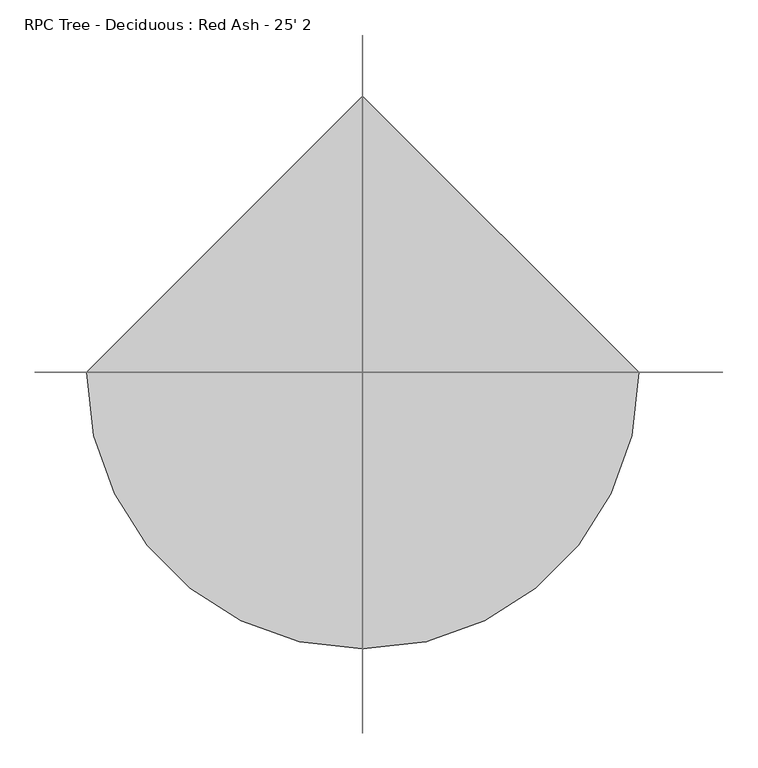
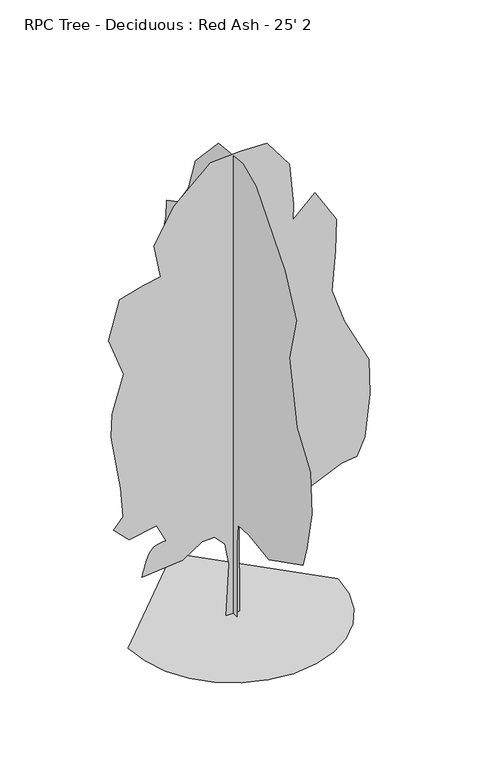
"""IFC4 building model written with IfcOpenShell, lengths in millimetres: geographic element geometry, RPC Tree - Deciduous : Red Ash - 25' 2."""

from ifc_helpers import new_model, si_unit, origin, place, context, project, spatial, triangles, source, transform, mapped, element, save


def rpc_tree_deciduous_red_ash_25_2_8bacb0ea(model_context):
    return source(origin(), model_context, "Body", "Tessellation", [
        triangles([(-460.5867119, 0.0, 1.73e-05), (-448.4102386, -105.5360182, 1.73e-05), (-413.73205, -202.4539578, 1.73e-05), (-359.3285757, -287.9770261, 1.73e-05), (-287.9770625, -359.3286484, 1.73e-05), (-202.4539215, -413.731941, 1.73e-05), (-105.5359728, -448.4102386, 1.73e-05), (2.01e-05, -460.5867119, 1.73e-05), (105.5360273, -448.4102749, 1.73e-05), (202.453976, -413.7320137, 1.73e-05), (287.9770625, -359.3285757, 1.73e-05), (359.328721, -287.9770625, 1.73e-05), (413.7319774, -202.4539033, 1.73e-05), (448.4102386, -105.5359456, 1.73e-05), (460.5867119, 4.03e-05, 1.73e-05), (-6.04e-05, 460.5867119, 1.73e-05), (-3e-06, -28.7969523, 0.0), (7e-06, -28.3490804, 334.4751509), (9e-06, -36.3669481, 430.5848368), (2e-07, -122.8711066, 436.286342), (-1.62e-05, -273.3895626, 413.9259336), (-3.93e-05, -533.0339613, 545.6295951), (-3.96e-05, -563.1376834, 643.4666828), (-3.81e-05, -600.7673269, 824.0887974), (-3.13e-05, -589.4785174, 1012.2369787), (-1.63e-05, -487.3069559, 1159.4848223), (-1.5e-06, -427.6716062, 1444.9777885), (-1e-06, -480.3526566, 1648.1777401), (1.34e-05, -393.8045963, 1828.8), (4.39e-05, -175.5528201, 2088.4444714), (5.56e-05, -76.4961938, 2133.0943623), (7.45e-05, 110.432449, 2114.7853054), (8.74e-05, 287.29173, 1926.6370514), (8.82e-05, 339.9732528, 1768.5926285), (9.3e-05, 418.9951735, 1655.7037342), (0.0001007, 505.5436698, 1610.5482056), (9.89e-05, 509.3066305, 1535.2888458), (9.87e-05, 531.8844312, 1448.7407856), (9.17e-05, 494.254824, 1347.1407372), (9.23e-05, 528.1214705, 1249.3038311), (9.18e-05, 561.9881169, 1113.8371725), (8.99e-05, 554.4622318, 1076.20742), (8.05e-05, 490.4918996, 985.89629), (7.64e-05, 486.4472337, 861.7184772), (7.37e-05, 482.9659055, 782.6962658), (7.12e-05, 486.7289025, 684.8593597), (6.75e-05, 490.4919359, 549.3927011), (6.08e-05, 437.8103768, 508.0000242), (5.06e-05, 339.9733981, 508.0000242), (5.12e-05, 385.1289631, 368.7704049), (4.8e-05, 377.5786245, 289.767669), (4.25e-05, 308.8486991, 343.7942041), (2.76e-05, 176.2495617, 309.8781421), (2.74e-05, 154.4793062, 379.977061), (1.76e-05, 60.4555758, 379.1207179), (1.41e-05, 36.6243452, 343.9336578), (9.2e-06, 22.273813, 229.1192815), (3.3e-06, 31.4064837, 3.6e-06), (-31.0438446, 1.4e-06, 1.25e-05), (-18.6792128, -2.7e-05, 233.3804677), (-36.2060431, -3.81e-05, 332.6241737), (-81.4206025, -4.2e-05, 382.2889475), (-135.418215, -3.94e-05, 380.4349909), (-222.9549776, -2.88e-05, 323.6148399), (-399.8142586, -1.93e-05, 308.5630334), (-397.3677873, -2.06e-05, 318.2941255), (-394.7567548, -2.19e-05, 328.3542672), (-391.8165999, -2.33e-05, 339.0726173), (-388.3827616, -2.48e-05, 350.7784799), (-384.2907148, -2.66e-05, 363.8005411), (-379.3758259, -2.85e-05, 378.4685411), (-373.4735699, -3.08e-05, 395.11113), (-366.0354338, -3.29e-05, 410.5469974), (-356.8200079, -3.47e-05, 421.8358795), (-346.1235314, -3.61e-05, 429.668868), (-334.2421709, -3.72e-05, 434.7374903), (-321.4722745, -3.81e-05, 437.7324019), (-308.1098634, -3.89e-05, 439.3450942), (-294.4512676, -3.96e-05, 440.2666586), (-335.8438173, -4.77e-05, 523.0518671), (-456.2587057, -3.97e-05, 500.4740664), (-523.991926, -4.48e-05, 568.2075047), (-482.5993581, -5.25e-05, 617.1259941), (-493.8882039, -6.81e-05, 752.5927254), (-535.2807718, -9.64e-05, 1004.7110573), (-531.574639, -0.000109, 1109.1263409), (-481.5768914, -0.0001313, 1277.7311657), (-546.5697267, -0.0001497, 1456.2666344), (-497.6511283, -0.0001725, 1629.3630455), (-396.0512252, -0.0001805, 1659.4665859), (-318.7556889, -0.0001855, 1673.1015095), (-347.1327722, -0.0002024, 1825.0370029), (-260.5845484, -0.0002246, 1979.3185741), (-98.777083, -0.0002491, 2126.0741512), (32.9265104, -0.0002558, 2133.6), (149.5784426, -0.0002604, 2129.8368576), (247.4154758, -0.000249, 1998.1334141), (265.4041852, -0.0002268, 1805.3050678), (262.8211307, -0.0002183, 1734.5915062), (360.3043156, -0.0002333, 1825.0370029), (454.3784062, -0.000219, 1670.7554317), (450.6154819, -0.0002015, 1525.0227573), (433.8480824, -0.0001792, 1344.1826328), (488.2450891, -0.0001626, 1185.3333172), (596.8939442, -0.0001419, 971.3754467), (600.3579042, -0.0001228, 809.9866785), (578.5561463, -9.89e-05, 617.1259214), (544.6894999, -8.8e-05, 538.10371), (476.9561342, -8.41e-05, 530.5777885), (345.252509, -7.12e-05, 470.3703444), (228.600545, -5.62e-05, 387.5852085), (72.0934329, -5.74e-05, 454.8792841), (26.0542441, -4.95e-05, 405.3377223), (29.1634679, -1.3e-06, 9.9e-06)], [[15, 16, 1], [14, 15, 1], [14, 1, 2], [13, 14, 2], [13, 2, 3], [13, 3, 4], [12, 13, 4], [11, 12, 4], [11, 4, 5], [11, 5, 6], [11, 6, 7], [11, 7, 8], [11, 8, 9], [11, 9, 10], [50, 51, 52], [57, 58, 17], [57, 17, 18], [56, 57, 18], [56, 18, 19], [55, 56, 19], [49, 50, 52], [52, 53, 54], [49, 52, 54], [35, 36, 37], [46, 47, 48], [46, 48, 49], [21, 22, 23], [20, 21, 23], [20, 23, 24], [20, 24, 25], [20, 25, 26], [19, 20, 26], [19, 26, 27], [45, 46, 49], [31, 32, 33], [30, 31, 33], [29, 30, 33], [29, 33, 34], [28, 29, 34], [27, 28, 34], [19, 27, 34], [19, 34, 35], [19, 35, 37], [19, 37, 38], [19, 38, 39], [19, 39, 40], [19, 40, 41], [19, 41, 42], [19, 42, 43], [19, 43, 44], [19, 44, 45], [19, 45, 49], [19, 49, 54], [55, 19, 54], [64, 65, 66], [64, 66, 67], [64, 67, 68], [99, 100, 101], [64, 68, 69], [64, 69, 70], [64, 70, 71], [114, 59, 60], [113, 114, 60], [113, 60, 61], [113, 61, 62], [64, 71, 72], [64, 72, 73], [64, 73, 74], [64, 74, 75], [64, 75, 76], [64, 76, 77], [64, 77, 78], [64, 78, 79], [63, 64, 79], [81, 82, 83], [80, 81, 83], [99, 101, 102], [107, 108, 109], [110, 111, 112], [88, 89, 90], [87, 88, 90], [87, 90, 91], [80, 83, 84], [95, 96, 97], [95, 97, 98], [94, 95, 98], [93, 94, 98], [92, 93, 98], [91, 92, 98], [91, 98, 99], [87, 91, 99], [87, 99, 102], [87, 102, 103], [87, 103, 104], [86, 87, 104], [85, 86, 104], [84, 85, 104], [80, 84, 104], [80, 104, 105], [80, 105, 106], [80, 106, 107], [80, 107, 109], [80, 109, 110], [80, 110, 112], [79, 80, 112], [63, 79, 112], [62, 63, 112], [113, 62, 112]], closed=False),
    ])


if __name__ == "__main__":
    model = new_model("IFC4")
    model_context = context("Model", 3, world=origin())
    ifc_project = project(units=[si_unit("LENGTHUNIT", "METRE", prefix="MILLI")], contexts=[model_context])
    site = spatial("IfcSite", under=ifc_project)
    building = spatial("IfcBuilding", under=site)
    placement = place(None, origin())
    rpc_tree_deciduous_red_ash_25_2_shape = rpc_tree_deciduous_red_ash_25_2_8bacb0ea(model_context)
    element("IfcGeographicElement", 1, ObjectType="RPC Tree - Deciduous : Red Ash - 25' 2", at=placement, inside=building, context=model_context, shape_type="MappedRepresentation", body=[
        mapped(rpc_tree_deciduous_red_ash_25_2_shape, transform((0.0, 0.0, 0.0), x_axis=(1.0, 0.0, 0.0), y_axis=(0.0, 1.0, 0.0), z_axis=(0.0, 0.0, 1.0))),
    ])
    save(model, "model.ifc")

# Revit data of these elements
# Type "RPC Tree - Deciduous : Red Ash - 25' 2"
#   built-in parameter 1005198 = "{2, 15},{22, RPC-8-G3GR-497X-PHW5-6},{1, 0},{1, 0},{2, 37},{1, 8},{5, Color},{1, 0},{1, 0},{3, 0.8},{3, 0.8},{3, 0.8},{1, 8},{7, BBoxMin},{1, 0},{1, 0},{1, 0},{1, 0},{1, 0},{1, 8},{7, BBoxMax},{1, 0},{1, 0},{1, 0},{1, 0},{1, 0},{2, 11},{9, RPCTypeId},{1, 0},{1, 0},{22, RPC-8-G3GR-497X-PHW5-6},{1, 6},{14, RPCPlantHeight},{1, 0},{1, 0},{2, 25},{2, 11},{7, keyword},{1, 0},{1, 0},{78, :Geometry:RPC:Red Ash:red ash:frainus pennsylvanica:frene rouge:deciduous:tree},{2, 11},{8, category},{1, 0},{1, 0},{16, :Trees [General]},{2, 11},{12, LocalizedUID},{1, 0},{1, 0},{7, Red Ash},{2, 14},{6, Height},{1, 0},{1, 0},{2, 25},{1, 2},{16, Cast Reflections},{1, 0},{1, 0},{1, 0},{1, 2},{6, Jitter},{1, 0},{1, 0},{1, 1},{1, 2},{9, Billboard},{1, 0},{1, 0},{1, 0},{1, 2},{12, Cast Shadows},{1, 0},{1, 0},{1, 1},{1, 2},{20, Apply Filter Effects},{1, 0},{1, 0},{1, 0},{2, 11},{28, Apply Filter Effects-Text-FC},{1, 0},{1, 0},{4, None},{2, 11},{20, AdvancedUIDefinition},{1, 0},{1, 0},{0, },{2, 11},{10, AssetLibID},{1, 0},{1, 0},{36, 4D3F6E72-3F99-4203-98E9-AF80B3C7A7A4},{2, 11},{10, BaseSchema},{1, 0},{1, 0},{9, RPCSchema},{2, 11},{12, ExchangeGUID},{1, 0},{1, 0},{0, },{1, 2},{6, Hidden},{1, 0},{1, 0},{1, 0},{1, 4},{11, RPCCategory},{1, 0},{1, 0},{1, 0},{2, 11},{8, RPCImage},{1, 0},{1, 0},{0, },{1, 4},{13, SchemaVersion},{1, 0},{1, 0},{1, 4},{2, 11},{12, UIDefinition},{1, 0},{1, 0},{0, },{2, 11},{6, UIName},{1, 0},{1, 0},{22, RPC-8-G3GR-497X-PHW5-6},{2, 11},{11, VersionGUID},{1, 0},{1, 0},{9, RPCSchema},{2, 11},{9, assettype},{1, 0},{1, 0},{11, RPCGeometry},{2, 11},{11, description},{1, 0},{1, 0},{0, },{2, 11},{9, localname},{1, 0},{1, 0},{3, RPC},{2, 11},{9, localtype},{1, 0},{1, 0},{3, RPC},{1, 4},{8, revision},{1, 0},{1, 0},{1, 1},{2, 11},{9, thumbnail},{1, 0},{1, 0},{0, },{1, 4},{7, version},{1, 0},{1, 0},{1, 1},{1, 2},{20, RPC_Cast Reflections},{1, 0},{1, 0},{1, 1},{1, 2},{10, RPC_Jitter},{1, 0},{1, 0},{1, 1},{1, 2},{13, RPC_Billboard},{1, 0},{1, 0},{1, 0},{1, 2},{16, RPC_Cast Shadows},{1, 0},{1, 0},{1, 1},{21, assetlibrary_base.fbx},{1, 5},"
#   built-in parameter 1005195 = "RPC-8-G3GR-497X-PHW5-6"
#   Type Comments = "Red Maple"
#   Assembly Code = "G2050500"
#   Height = 7' - 0"
#   Default Elevation = 0
